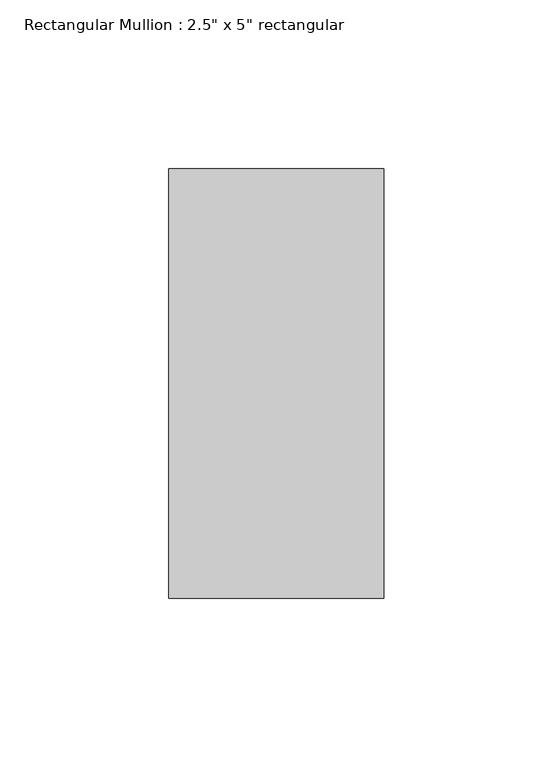
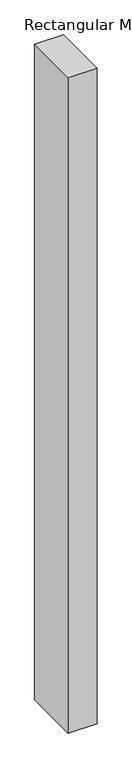
"""IFC4 building model written with IfcOpenShell, lengths in millimetres: member geometry."""

from ifc_helpers import new_model, si_unit, frame, origin, place, context, project, spatial, polyline, outline, extrude, source, transform, mapped, element, save


def member_82905deb(model_context):
    return source(origin(), model_context, "Body", "SweptSolid", [
        extrude(outline(polyline([(31.75, 63.5), (31.75, -63.5), (-31.75, -63.5), (-31.75, 63.5), (31.75, 63.5)])), frame((0.0, 0.0, -1524.0), z_axis=(0.0, 0.0, 1.0), x_axis=(1.0, 0.0, 0.0)), (0.0, 0.0, 1.0), 1524.0),
    ])


if __name__ == "__main__":
    model = new_model("IFC4")
    model_context = context("Model", 3, world=origin())
    ifc_project = project(units=[si_unit("LENGTHUNIT", "METRE", prefix="MILLI")], contexts=[model_context])
    site = spatial("IfcSite", under=ifc_project)
    building = spatial("IfcBuilding", under=site)
    placement = place(None, origin())
    member_shape = member_82905deb(model_context)
    element("IfcMember", 1, ObjectType="Rectangular Mullion : 2.5\" x 5\" rectangular", at=placement, inside=building, context=model_context, shape_type="MappedRepresentation", body=[
        mapped(member_shape, transform((0.0, 0.0, 0.0), x_axis=(1.0, 0.0, 0.0), y_axis=(0.0, 1.0, 0.0), z_axis=(0.0, 0.0, 1.0))),
    ])
    save(model, "model.ifc")

# Revit data of these elements
# Type "Rectangular Mullion : 2.5\" x 5\" rectangular"
#   built-in parameter 1007304 = 0.416667 (stored number, unit not read)
#   built-in parameter 1007301 = 0.104167 (stored number, unit not read)
#   built-in parameter 1007300 = 0.104167 (stored number, unit not read)
# Element 1 (IfcMember, "Rectangular Mullion : 2.5\" x 5\" rectangular")
#   Materials on its faces: "metal black"
# Materials
#   "metal black": class "Generic", colour RGB 120 120 120, transparency 0, Cost = 0
